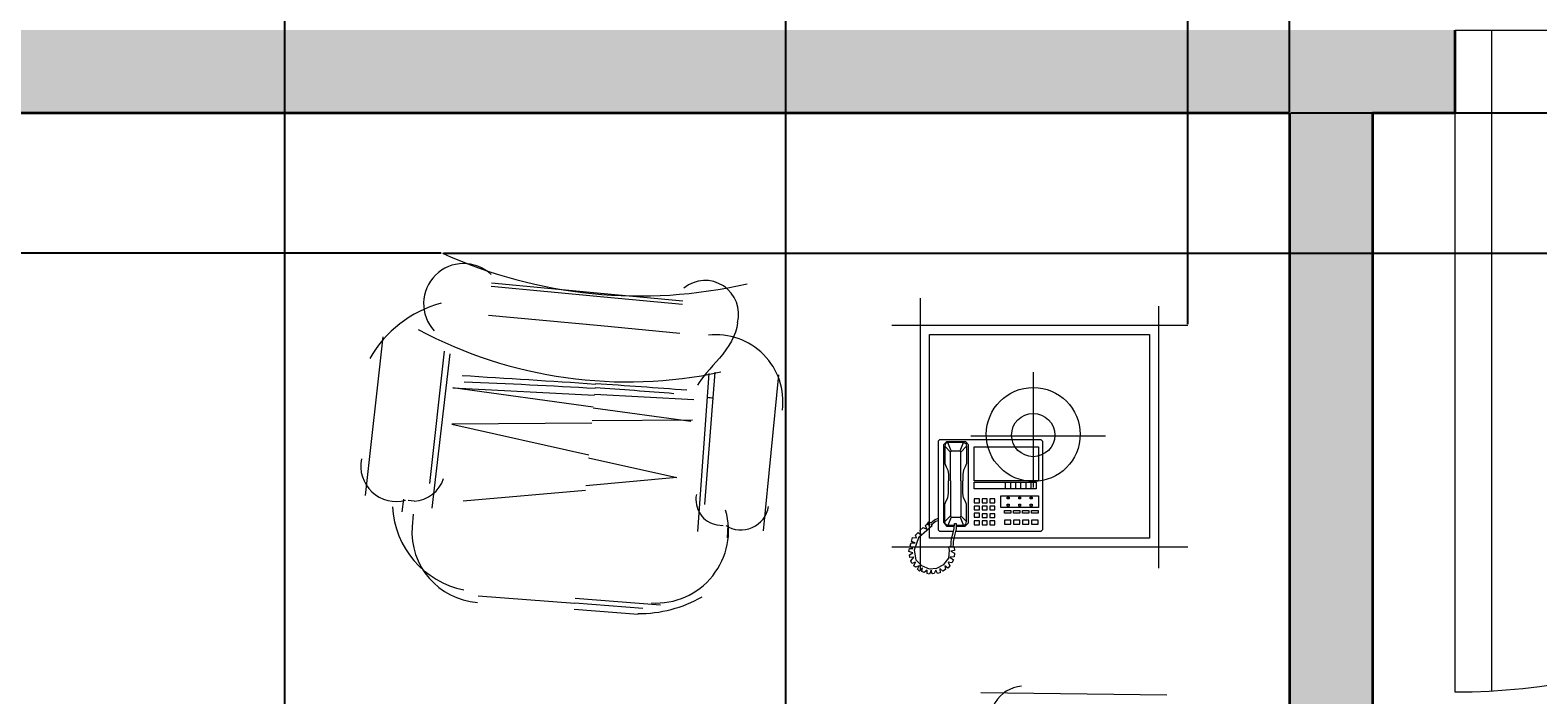
# Model space of a CAD drawing. Units: inches. Extents: x 2807 to 3326, y 2005 to 2580.
# Tile 6 of 12: x 3067 to 3149, y 2243 to 2280. Entities that reach past the tile are written whole.
import ezdxf

# ---------------------------------------------------------------- set-up
doc = ezdxf.new("R2010")
doc.units = ezdxf.units.IN
doc.header["$LTSCALE"] = 0.4
for name, color, linetype, lineweight in [('A-ANNO-DIMS', 2, 'Continuous', 18), ('A-WALL-PATT', 231, 'Continuous', 13), ('DOORS', 144, 'Continuous', 18), ('Furniture', 7, 'Continuous', 15), ('WALL', 233, 'Continuous', 35)]:
    doc.layers.add(name, color=color, linetype=linetype, lineweight=lineweight)
doc.styles.get("Standard").update_dxf_attribs({"font": 'txt', "height": 5})
doc.dimstyles.get("Standard").update_dxf_attribs({"dimtxt": 0.18, "dimasz": 0.18, "dimexe": 0.18, "dimexo": 0.0625, "dimgap": 0.09, "dimtad": 0, "dimtih": 1, "dimtoh": 1, "dimdec": 4, "dimzin": 0, "dimdsep": 46, "dimtxsty": 'Standard', "dimcen": 0.09, "dimadec": 0, "dimazin": 0, "dimtfac": 1, "dimtdec": 4, "dimtofl": 0, "dimtmove": 0, "dimatfit": 3, "dimfxl": 1, "dimtolj": 1, "dimtzin": 0, "dimarcsym": 0})

# ---------------------------------------------------------------- blocks, each defined once
blk = doc.blocks.new('DOOR-36')
for p, q in [((0, 0), (-36, 0)), ((-2, -35.944), (-2, 0)), ((0, -36), (0, 0))]:
    blk.add_line(p, q)
blk.add_arc((0, 0), 36, 180, 270)
blk = doc.blocks.new('*D61')
at = {"layer": 'A-ANNO-DIMS', "color": 0, "lineweight": -2, "ltscale": 0.4, "transparency": 16777216}
for p, q in [((3088.922898, 2267.452063), (2816.937191, 2267.452063)), ((2817.117191, 2267.272063), (2817.117191, 2223.175564)), ((2817.117191, 2173.899065), (2817.117191, 2217.995564)), ((3079.479513, 2173.719065), (2816.937191, 2173.719065))]:
    blk.add_line(p, q, dxfattribs=at)
at = {"layer": 'A-ANNO-DIMS', "color": 0, "ltscale": 0.4, "transparency": 16777216}
for points in [[(2817.087191, 2267.272063), (2817.147191, 2267.272063), (2817.117191, 2267.452063)], [(2817.087191, 2173.899065), (2817.147191, 2173.899065), (2817.117191, 2173.719065)]]:
    blk.add_solid(points, dxfattribs=at)
at = {"layer": 'Defpoints', "color": 0, "ltscale": 0.4, "transparency": 16777216}
for p in [(2817.117191, 2267.452063), (3088.985398, 2267.452063), (3079.542013, 2173.719065)]:
    blk.add_point(p, dxfattribs=at)
at = {"layer": 'A-ANNO-DIMS', "color": 0, "ltscale": 0.4, "transparency": 16777216, "insert": (2817.117191, 2220.585564), "char_height": 5, "attachment_point": 5}
blk.add_mtext('\\A1;93.73', dxfattribs=at)
blk = doc.blocks.new('*D64')
at = {"layer": 'A-ANNO-DIMS', "color": 0, "lineweight": -2, "ltscale": 0.4, "transparency": 16777216}
for p, q in [((3080.426, 2237.614), (3080.426, 2577.206)), ((3080.606, 2577.026), (3081.577, 2577.026)), ((3107.489, 2577.026), (3106.519, 2577.026)), ((3107.669, 2237.614), (3107.669, 2577.206))]:
    blk.add_line(p, q, dxfattribs=at)
at = {"layer": 'A-ANNO-DIMS', "color": 0, "ltscale": 0.4, "transparency": 16777216}
for points in [[(3080.606, 2577.056), (3080.606, 2576.996), (3080.426, 2577.026)], [(3107.489, 2577.056), (3107.489, 2576.996), (3107.669, 2577.026)]]:
    blk.add_solid(points, dxfattribs=at)
at = {"layer": 'Defpoints', "color": 0, "ltscale": 0.4, "transparency": 16777216}
for p in [(3107.669, 2577.026), (3080.426, 2237.552), (3107.669, 2237.552)]:
    blk.add_point(p, dxfattribs=at)
at = {"layer": 'A-ANNO-DIMS', "color": 0, "ltscale": 0.4, "transparency": 16777216, "insert": (3094.048, 2577.026), "char_height": 5, "attachment_point": 5}
blk.add_mtext('\\A1;27.243', dxfattribs=at)
blk = doc.blocks.new('*D66')
at = {"layer": 'A-ANNO-DIMS', "color": 0, "lineweight": -2, "ltscale": 0.4, "transparency": 16777216}
for p, q in [((3129.534988, 2263.581941), (3129.534988, 2577.206496)), ((3129.714988, 2577.026496), (3134.887191, 2577.026496)), ((3135.067191, 2275.138996), (3135.067191, 2577.206496)), ((3135.067191, 2577.026496), (3135.247191, 2577.026496))]:
    blk.add_line(p, q, dxfattribs=at)
at = {"layer": 'A-ANNO-DIMS', "color": 0, "ltscale": 0.4, "transparency": 16777216}
for points in [[(3129.714988, 2577.056496), (3129.714988, 2576.996496), (3129.534988, 2577.026496)], [(3134.887191, 2577.056496), (3134.887191, 2576.996496), (3135.067191, 2577.026496)]]:
    blk.add_solid(points, dxfattribs=at)
at = {"layer": 'Defpoints', "color": 0, "ltscale": 0.4, "transparency": 16777216}
for p in [(3135.067191, 2577.026496), (3135.067191, 2275.076496), (3129.534988, 2263.519441)]:
    blk.add_point(p, dxfattribs=at)
at = {"layer": 'A-ANNO-DIMS', "color": 0, "ltscale": 0.4, "transparency": 16777216, "insert": (3145.337191, 2577.026496), "char_height": 5, "attachment_point": 5}
blk.add_mtext('\\A1;5.532', dxfattribs=at)
blk = doc.blocks.new('*D67')
at = {"layer": 'A-ANNO-DIMS', "color": 0, "lineweight": -2, "ltscale": 0.4, "transparency": 16777216}
for p, q in [((3135.13, 2275.076), (3316.197, 2275.076)), ((3316.017, 2274.896), (3316.017, 2273.854)), ((3316.017, 2267.632), (3316.017, 2268.674)), ((3089.048, 2267.452), (3316.197, 2267.452))]:
    blk.add_line(p, q, dxfattribs=at)
at = {"layer": 'A-ANNO-DIMS', "color": 0, "ltscale": 0.4, "transparency": 16777216}
for points in [[(3315.987, 2274.896), (3316.047, 2274.896), (3316.017, 2275.076)], [(3315.987, 2267.632), (3316.047, 2267.632), (3316.017, 2267.452)]]:
    blk.add_solid(points, dxfattribs=at)
at = {"layer": 'Defpoints', "color": 0, "ltscale": 0.4, "transparency": 16777216}
for p in [(3135.067, 2275.076), (3088.985, 2267.452), (3316.017, 2267.452)]:
    blk.add_point(p, dxfattribs=at)
at = {"layer": 'A-ANNO-DIMS', "color": 0, "ltscale": 0.4, "transparency": 16777216, "insert": (3316.017, 2271.264), "char_height": 5, "attachment_point": 5}
blk.add_mtext('\\A1;7.624', dxfattribs=at)
blk = doc.blocks.new('*D72')
at = {"layer": 'A-ANNO-DIMS', "color": 0, "lineweight": -2, "ltscale": 0.4, "transparency": 16777216}
for p, q in [((2948.067, 2279.639), (2948.067, 2307.206)), ((2948.247, 2307.026), (3060.049, 2307.026)), ((3184.887, 2307.026), (3073.086, 2307.026)), ((3185.067, 2279.639), (3185.067, 2307.206))]:
    blk.add_line(p, q, dxfattribs=at)
at = {"layer": 'A-ANNO-DIMS', "color": 0, "ltscale": 0.4, "transparency": 16777216}
for points in [[(2948.247, 2307.056), (2948.247, 2306.996), (2948.067, 2307.026)], [(3184.887, 2307.056), (3184.887, 2306.996), (3185.067, 2307.026)]]:
    blk.add_solid(points, dxfattribs=at)
at = {"layer": 'Defpoints', "color": 0, "ltscale": 0.4, "transparency": 16777216}
for p in [(3185.067, 2307.026), (2948.067, 2279.576), (3185.067, 2279.576)]:
    blk.add_point(p, dxfattribs=at)
at = {"layer": 'A-ANNO-DIMS', "color": 0, "ltscale": 0.4, "transparency": 16777216, "insert": (3066.567, 2307.026), "char_height": 5, "attachment_point": 5}
blk.add_mtext('\\A1;237', dxfattribs=at)

msp = doc.modelspace()

# ---------------------------------------------------------------- hatches: boundary and pattern name
at = {"layer": 'A-WALL-PATT', "ltscale": 0.4}
h = msp.add_hatch(color=256, dxfattribs=at)
h.dxf.hatch_style = 1
h.paths.add_polyline_path([(3288.5672, 2549.5765), (2941.5672, 2549.5765), (2941.5672, 2540.5765), (2993.5672, 2540.5765), (2993.5672, 2489.5693), (2998.0672, 2489.5693), (2998.0672, 2540.5765), (3135.0672, 2540.5765), (3135.0672, 2479.0765), (3139.5672, 2479.0765), (3139.5672, 2540.5765), (3279.5672, 2540.5765), (3279.5672, 2510.5765), (3288.5672, 2510.5765)])
h.paths.add_polyline_path([(2905.5672, 2549.5765), (2844.5672, 2549.5765), (2844.5672, 2445.94), (2853.5672, 2445.94), (2853.5672, 2540.5765), (2905.5672, 2540.5765)])
h.paths.add_polyline_path([(2853.5672, 2409.94), (2844.5672, 2409.94), (2844.5672, 2371.3497), (2853.5672, 2371.3497), (2853.5672, 2380.0765), (2909.0672, 2380.0765), (2909.0672, 2384.5765), (2853.5672, 2384.5765)])
h.paths.add_polyline_path([(2998.0672, 2389.0765), (2993.5672, 2389.0765), (2993.5672, 2384.5765), (2939.0672, 2384.5765), (2939.0672, 2380.0765), (2943.5672, 2380.0765), (2943.5672, 2314.0765), (2948.0672, 2314.0765), (2948.0672, 2380.0765), (2998.0672, 2380.0765)])
h.paths.add_polyline_path([(2998.0672, 2471.8029), (2993.5672, 2471.8029), (2993.5672, 2425.0765), (2998.0672, 2425.0765)])
h.paths.add_polyline_path([(2953.0672, 2279.5765), (2948.0672, 2279.5765), (2948.0672, 2284.0765), (2943.5672, 2284.0765), (2943.5672, 2279.5765), (2853.5672, 2279.5765), (2853.5672, 2289.0663), (2844.5672, 2289.0663), (2844.5672, 2227.8961), (2853.5672, 2227.8961), (2853.5672, 2275.0765), (2953.0672, 2275.0765)])
h.paths.add_polyline_path([(2943.5672, 2332.0765), (2853.5672, 2332.0765), (2853.5672, 2347.3497), (2844.5672, 2347.3497), (2844.5672, 2313.0663), (2853.5672, 2313.0663), (2853.5672, 2327.5765), (2943.5672, 2327.5765)])
h.paths.add_polyline_path([(3144.0672, 2279.5765), (2993.5672, 2279.5765), (2989.0672, 2279.5765), (2989.0672, 2275.0765), (2993.5672, 2275.0765), (2993.5672, 2144.5765), (2984.5672, 2144.5765), (2984.5672, 2135.5765), (2993.5672, 2135.5765), (2993.5672, 2120.0765), (3036.5672, 2120.0765), (3036.5672, 2129.0765), (2998.0672, 2129.0765), (2998.0672, 2275.0765), (3135.0672, 2275.0765), (3135.0672, 2129.0765), (3096.5672, 2129.0765), (3096.5672, 2120.0765), (3139.5672, 2120.0765), (3139.5672, 2135.5765), (3148.5672, 2135.5765), (3148.5672, 2144.5765), (3139.5672, 2144.5765), (3139.5672, 2275.0765), (3144.0672, 2275.0765)])
h.paths.add_polyline_path([(2984.5672, 2144.5765), (2925.9914, 2144.5765), (2925.9914, 2135.5765), (2984.5672, 2135.5765)])
h.paths.add_polyline_path([(2889.9914, 2144.5765), (2853.5672, 2144.5765), (2853.5672, 2191.8961), (2844.5672, 2191.8961), (2844.5672, 2135.5765), (2889.9914, 2135.5765)])
h.paths.add_polyline_path([(3196.0672, 2144.5765), (3148.5672, 2144.5765), (3148.5672, 2135.5765), (3196.0672, 2135.5765)])
h.paths.add_polyline_path([(3288.5672, 2191.8265), (3279.5672, 2191.8265), (3279.5672, 2144.5765), (3232.0672, 2144.5765), (3232.0672, 2135.5765), (3288.5672, 2135.5765)])
h.paths.add_polyline_path([(3288.5672, 2292.8229), (3279.5672, 2292.8229), (3279.5672, 2291.4371), (3279.5672, 2279.5765), (3189.5672, 2279.5765), (3189.5672, 2293.0765), (3185.0672, 2293.0765), (3185.0672, 2279.5765), (3180.0672, 2279.5765), (3180.0672, 2275.0765), (3279.5672, 2275.0765), (3279.5672, 2227.8265), (3288.5672, 2227.8265)])
h.paths.add_polyline_path([(3288.5672, 2368.0765), (3279.5672, 2368.0765), (3279.5672, 2332.0765), (3174.0672, 2332.0765), (3174.0672, 2327.5765), (3185.0672, 2327.5765), (3189.5672, 2327.5765), (3279.5672, 2327.5765), (3279.5672, 2316.8229), (3288.5672, 2316.8229)])
h.paths.add_polyline_path([(3288.5672, 2474.5765), (3279.5672, 2474.5765), (3279.5672, 2444.5765), (3139.5672, 2444.5765), (3139.5672, 2449.0765), (3135.0672, 2449.0765), (3135.0672, 2327.5765), (3144.0672, 2327.5765), (3144.0672, 2332.0765), (3139.5672, 2332.0765), (3139.5672, 2440.0765), (3279.5672, 2440.0765), (3279.5672, 2404.0765), (3288.5672, 2404.0765)])

# ---------------------------------------------------------------- linework, layer by layer
at = {"layer": 'Furniture'}
for p, q in [((3091.6497, 2265.6621), (3097.7622, 2265.0849)), ((3091.6663, 2265.8372), (3097.7788, 2265.2599)), ((3097.7622, 2265.0849), (3102.0439, 2264.6805)), ((3097.7788, 2265.2599), (3102.0604, 2264.8555)), ((3114.9915, 2250.2169), (3114.9915, 2265.011)), ((3091.5009, 2264.0867), (3097.6134, 2263.5094)), ((3127.942, 2264.5759), (3127.942, 2250.3256)), ((3097.6134, 2263.5094), (3101.8951, 2263.1051)), ((3129.535, 2263.5194), (3113.4239, 2263.5194)), ((3084.8134, 2254.2733), (3085.7585, 2262.9082)), ((3115.4812, 2263.0297), (3127.4523, 2263.0297)), ((3115.4812, 2251.9543), (3115.4812, 2263.0297)), ((3127.4523, 2263.0297), (3127.4523, 2251.9543)), ((3088.3068, 2254.9333), (3089.1099, 2262.121)), ((3088.4292, 2253.5908), (3089.4174, 2261.9813)), ((3102.8876, 2252.3217), (3103.4976, 2260.9089)), ((3103.2691, 2253.7776), (3103.8258, 2260.9885)), ((3107.2595, 2260.8432), (3106.4335, 2252.3569)), ((3121.1232, 2260.9852), (3121.1232, 2254.7047)), ((3097.1952, 2259.0813), (3089.5637, 2260.1318)), ((3089.5637, 2260.1318), (3097.2557, 2259.7216)), ((3097.261, 2259.7772), (3102.6702, 2259.4888)), ((3102.584, 2258.3728), (3097.125, 2258.3374)), ((3102.4914, 2258.2936), (3097.1898, 2259.0233)), ((3097.112, 2258.2001), (3089.4972, 2258.1507)), ((3089.4972, 2258.1507), (3096.9502, 2256.4868)), ((3117.7287, 2257.5259), (3125.0556, 2257.5259)), ((3116.029, 2257.3022), (3115.959, 2257.2323)), ((3115.959, 2257.2323), (3115.959, 2252.4042)), ((3121.5568, 2257.3022), (3116.029, 2257.3022)), ((3116.4138, 2257.1973), (3116.2389, 2257.0223)), ((3116.2389, 2257.0223), (3116.2389, 2252.824)), ((3116.3438, 2257.0923), (3116.3089, 2256.9524)), ((3116.3089, 2256.9524), (3116.6237, 2256.6375)), ((3116.3089, 2256.9524), (3116.3089, 2256.0077)), ((3116.4838, 2257.1623), (3116.3438, 2257.0923)), ((3117.4634, 2257.1973), (3116.4138, 2257.1973)), ((3116.6587, 2256.7075), (3116.4838, 2257.1623)), ((3117.3235, 2257.1623), (3116.4838, 2257.1623)), ((3116.6237, 2256.6375), (3116.6587, 2256.7075)), ((3116.6587, 2256.7075), (3117.1485, 2256.7075)), ((3117.1485, 2256.7075), (3117.3235, 2257.1623)), ((3117.1835, 2256.6375), (3117.1485, 2256.7075)), ((3117.4984, 2256.9524), (3117.1835, 2256.6375)), ((3117.3235, 2257.1623), (3117.4634, 2257.0923)), ((3117.6034, 2257.0223), (3117.4634, 2257.1973)), ((3117.4634, 2257.0923), (3117.4984, 2256.9524)), ((3117.4984, 2256.9524), (3117.4984, 2256.0077)), ((3117.6034, 2252.789), (3117.6034, 2257.0223)), ((3117.9182, 2256.9174), (3121.4169, 2256.9174)), ((3117.9182, 2255.0631), (3117.9182, 2256.9174)), ((3121.4169, 2256.9174), (3121.4169, 2255.0631)), ((3121.5568, 2257.3022), (3121.6268, 2257.2323)), ((3121.6268, 2257.2323), (3121.6268, 2252.4042)), ((3096.934, 2256.3153), (3101.7371, 2255.243)), ((3116.3089, 2256.0077), (3116.3788, 2255.8328)), ((3116.3788, 2255.8328), (3116.4838, 2255.6579)), ((3116.6237, 2255.0631), (3116.6237, 2256.6375)), ((3117.1835, 2255.0631), (3117.1835, 2256.6375)), ((3117.4284, 2255.8328), (3117.3235, 2255.6579)), ((3117.4984, 2256.0077), (3117.4284, 2255.8328)), ((3101.7371, 2255.243), (3096.7911, 2254.8017)), ((3116.4838, 2255.6579), (3116.5188, 2255.413)), ((3116.5188, 2255.413), (3116.5188, 2255.0631)), ((3116.5188, 2254.3984), (3116.5188, 2255.0631)), ((3116.6237, 2255.0631), (3116.6237, 2253.1739)), ((3117.1835, 2255.0631), (3117.1835, 2253.1739)), ((3117.3235, 2255.6579), (3117.2885, 2255.413)), ((3117.2885, 2255.413), (3117.2885, 2255.0631)), ((3117.2885, 2254.3984), (3117.2885, 2255.0631)), ((3121.4169, 2255.0631), (3117.9182, 2255.0631)), ((3096.7673, 2254.5499), (3090.1246, 2253.9572)), ((3116.4838, 2254.1535), (3116.5188, 2254.3984)), ((3117.3235, 2254.1535), (3117.2885, 2254.3984)), ((3117.9182, 2254.9931), (3121.2769, 2254.9931)), ((3117.9182, 2254.6433), (3117.9182, 2254.9931)), ((3121.2769, 2254.6433), (3117.9182, 2254.6433)), ((3119.3527, 2254.2584), (3121.4169, 2254.2584)), ((3119.3527, 2253.6287), (3119.3527, 2254.2584)), ((3119.5976, 2254.9931), (3119.5976, 2254.6433)), ((3119.7025, 2254.0835), (3119.7025, 2254.1885)), ((3119.7025, 2254.1885), (3119.8075, 2254.1885)), ((3119.8075, 2254.1885), (3119.8075, 2254.0835)), ((3119.8775, 2254.9931), (3119.8775, 2254.6433)), ((3120.1573, 2254.9931), (3120.1573, 2254.6433)), ((3120.3323, 2254.0835), (3120.3323, 2254.1885)), ((3120.3323, 2254.1885), (3120.4372, 2254.1885)), ((3120.4372, 2254.9931), (3120.4372, 2254.6433)), ((3120.4372, 2254.1885), (3120.4372, 2254.0835)), ((3120.7171, 2254.9931), (3120.7171, 2254.6433)), ((3120.962, 2254.1885), (3121.067, 2254.1885)), ((3120.962, 2254.0835), (3120.962, 2254.1885)), ((3120.997, 2254.9931), (3120.997, 2254.6433)), ((3121.067, 2254.1885), (3121.067, 2254.0835)), ((3121.2769, 2254.9931), (3121.2769, 2254.6433)), ((3121.4169, 2254.2584), (3121.4169, 2253.6287)), ((3086.8672, 2254.069), (3086.7887, 2253.3893)), ((3087.458, 2253.9711), (3087.1278, 2254.0092)), ((3116.3089, 2253.8036), (3116.3788, 2253.9785)), ((3116.3089, 2252.859), (3116.3089, 2253.8036)), ((3116.3788, 2253.9785), (3116.4838, 2254.1535)), ((3117.4284, 2253.9785), (3117.3235, 2254.1535)), ((3117.4984, 2253.8036), (3117.4284, 2253.9785)), ((3117.4984, 2252.859), (3117.4984, 2253.8036)), ((3118.1981, 2254.0835), (3117.9182, 2254.0835)), ((3117.9182, 2254.0835), (3117.9182, 2253.8736)), ((3117.9182, 2253.8736), (3118.1981, 2253.8736)), ((3117.9182, 2253.6986), (3117.9182, 2253.4887)), ((3118.1981, 2253.6986), (3117.9182, 2253.6986)), ((3117.9182, 2253.4887), (3118.1981, 2253.4887)), ((3118.1981, 2253.8736), (3118.1981, 2254.0835)), ((3118.1981, 2253.4887), (3118.1981, 2253.6986)), ((3118.3381, 2254.0835), (3118.3381, 2253.8736)), ((3118.618, 2254.0835), (3118.3381, 2254.0835)), ((3118.3381, 2253.8736), (3118.618, 2253.8736)), ((3118.3381, 2253.6986), (3118.3381, 2253.4887)), ((3118.618, 2253.6986), (3118.3381, 2253.6986)), ((3118.3381, 2253.4887), (3118.618, 2253.4887)), ((3118.618, 2253.8736), (3118.618, 2254.0835)), ((3118.618, 2253.4887), (3118.618, 2253.6986)), ((3119.0378, 2254.0835), (3118.7579, 2254.0835)), ((3118.7579, 2254.0835), (3118.7579, 2253.8736)), ((3118.7579, 2253.8736), (3119.0378, 2253.8736)), ((3118.7579, 2253.6986), (3118.7579, 2253.4887)), ((3119.0378, 2253.6986), (3118.7579, 2253.6986)), ((3118.7579, 2253.4887), (3119.0378, 2253.4887)), ((3119.0378, 2253.8736), (3119.0378, 2254.0835)), ((3119.0378, 2253.4887), (3119.0378, 2253.6986)), ((3121.4169, 2253.6287), (3119.3527, 2253.6287)), ((3119.5626, 2253.3138), (3119.5626, 2253.4537)), ((3119.5626, 2253.4537), (3119.9124, 2253.4537)), ((3119.8075, 2254.0835), (3119.7025, 2254.0835)), ((3119.7025, 2253.6986), (3119.7025, 2253.8036)), ((3119.7025, 2253.8036), (3119.8075, 2253.8036)), ((3119.8075, 2253.6986), (3119.7025, 2253.6986)), ((3119.8075, 2253.8036), (3119.8075, 2253.6986)), ((3119.9124, 2253.4537), (3119.9124, 2253.3138)), ((3120.0524, 2253.4537), (3120.4023, 2253.4537)), ((3120.0524, 2253.3138), (3120.0524, 2253.4537)), ((3120.4372, 2254.0835), (3120.3323, 2254.0835)), ((3120.3323, 2253.6986), (3120.3323, 2253.8036)), ((3120.3323, 2253.8036), (3120.4372, 2253.8036)), ((3120.4372, 2253.6986), (3120.3323, 2253.6986)), ((3120.4023, 2253.4537), (3120.4023, 2253.3138)), ((3120.4372, 2253.8036), (3120.4372, 2253.6986)), ((3120.5422, 2253.4537), (3120.8921, 2253.4537)), ((3120.5422, 2253.3138), (3120.5422, 2253.4537)), ((3120.8921, 2253.4537), (3120.8921, 2253.3138)), ((3121.067, 2254.0835), (3120.962, 2254.0835)), ((3120.962, 2253.6986), (3120.962, 2253.8036)), ((3120.962, 2253.8036), (3121.067, 2253.8036)), ((3121.067, 2253.6986), (3120.962, 2253.6986)), ((3121.032, 2253.4537), (3121.3819, 2253.4537)), ((3121.032, 2253.3138), (3121.032, 2253.4537)), ((3121.067, 2253.8036), (3121.067, 2253.6986)), ((3121.3819, 2253.4537), (3121.3819, 2253.3138)), ((3087.3925, 2253.2551), (3087.3422, 2252.5728)), ((3087.3925, 2253.2551), (3087.3422, 2252.5728)), ((3103.9227, 2252.6735), (3104.2542, 2252.6491)), ((3104.5214, 2252.6591), (3104.4712, 2251.9768)), ((3115.256, 2252.6413), (3115.3485, 2252.74)), ((3115.33, 2252.4379), (3115.256, 2252.6413)), ((3115.6258, 2252.6228), (3115.3423, 2252.37)), ((3115.3485, 2252.74), (3115.4347, 2252.6722)), ((3115.3854, 2252.777), (3115.4471, 2252.8387)), ((3115.4347, 2252.6722), (3115.3854, 2252.777)), ((3115.4471, 2252.8387), (3115.5765, 2252.7893)), ((3115.5518, 2252.6968), (3115.6258, 2252.6228)), ((3115.6258, 2252.6907), (3115.5518, 2252.6968)), ((3115.5765, 2252.7893), (3115.6504, 2252.8572)), ((3115.6627, 2252.74), (3115.6258, 2252.6907)), ((3115.6504, 2252.8572), (3115.749, 2252.9558)), ((3115.8045, 2252.851), (3115.6627, 2252.74)), ((3115.749, 2252.9558), (3115.959, 2253.0339)), ((3115.959, 2252.894), (3115.8045, 2252.851)), ((3116.2389, 2252.824), (3116.4138, 2252.6141)), ((3116.3089, 2252.859), (3116.6237, 2253.1739)), ((3116.3438, 2252.719), (3116.3089, 2252.859)), ((3116.4838, 2252.6491), (3116.3438, 2252.719)), ((3116.4138, 2252.6141), (3116.8235, 2252.6141)), ((3116.6587, 2253.1039), (3116.4838, 2252.6491)), ((3116.8261, 2252.6491), (3116.4838, 2252.6491)), ((3116.6237, 2253.1739), (3116.6587, 2253.1039)), ((3116.6587, 2253.1039), (3117.1485, 2253.1039)), ((3116.8134, 2252.4736), (3116.8337, 2252.754)), ((3116.8337, 2252.754), (3116.9386, 2252.754)), ((3116.9386, 2252.754), (3116.9337, 2252.4523)), ((3116.9363, 2252.6141), (3117.4284, 2252.6141)), ((3117.3235, 2252.6491), (3116.9369, 2252.6491)), ((3117.1835, 2253.1739), (3117.1485, 2253.1039)), ((3117.1485, 2253.1039), (3117.3235, 2252.6491)), ((3117.4984, 2252.859), (3117.1835, 2253.1739)), ((3117.3235, 2252.6491), (3117.4634, 2252.719)), ((3117.4284, 2252.6141), (3117.6034, 2252.789)), ((3117.4634, 2252.719), (3117.4984, 2252.859)), ((3118.1981, 2253.3138), (3117.9182, 2253.3138)), ((3117.9182, 2253.3138), (3117.9182, 2253.1039)), ((3117.9182, 2253.1039), (3118.1981, 2253.1039)), ((3118.1981, 2252.894), (3117.9182, 2252.894)), ((3117.9182, 2252.894), (3117.9182, 2252.684)), ((3117.9182, 2252.684), (3118.1981, 2252.684)), ((3118.1981, 2253.1039), (3118.1981, 2253.3138)), ((3118.1981, 2252.684), (3118.1981, 2252.894)), ((3118.618, 2253.2788), (3118.3381, 2253.2788)), ((3118.3381, 2253.2788), (3118.3381, 2253.0689)), ((3118.3381, 2253.0689), (3118.618, 2253.0689)), ((3118.618, 2252.894), (3118.3381, 2252.894)), ((3118.3381, 2252.894), (3118.3381, 2252.684)), ((3118.3381, 2252.684), (3118.618, 2252.684)), ((3118.618, 2253.0689), (3118.618, 2253.2788)), ((3118.618, 2252.684), (3118.618, 2252.894)), ((3119.0378, 2253.2788), (3118.7579, 2253.2788)), ((3118.7579, 2253.2788), (3118.7579, 2253.0689)), ((3118.7579, 2253.0689), (3119.0378, 2253.0689)), ((3119.0378, 2252.894), (3118.7579, 2252.894)), ((3118.7579, 2252.894), (3118.7579, 2252.684)), ((3118.7579, 2252.684), (3119.0378, 2252.684)), ((3119.0378, 2253.0689), (3119.0378, 2253.2788)), ((3119.0378, 2252.684), (3119.0378, 2252.894)), ((3119.9124, 2253.3138), (3119.5626, 2253.3138)), ((3119.9124, 2252.929), (3119.5626, 2252.929)), ((3119.5626, 2252.929), (3119.5626, 2252.719)), ((3119.5626, 2252.719), (3119.9124, 2252.719)), ((3119.9124, 2252.719), (3119.9124, 2252.929)), ((3120.4023, 2253.3138), (3120.0524, 2253.3138)), ((3120.0524, 2252.929), (3120.0524, 2252.719)), ((3120.4023, 2252.929), (3120.0524, 2252.929)), ((3120.0524, 2252.719), (3120.4023, 2252.719)), ((3120.4023, 2252.719), (3120.4023, 2252.929)), ((3120.8921, 2253.3138), (3120.5422, 2253.3138)), ((3120.5422, 2252.929), (3120.5422, 2252.719)), ((3120.8921, 2252.929), (3120.5422, 2252.929)), ((3120.5422, 2252.719), (3120.8921, 2252.719)), ((3120.8921, 2252.719), (3120.8921, 2252.929)), ((3121.3819, 2253.3138), (3121.032, 2253.3138)), ((3121.032, 2252.929), (3121.032, 2252.719)), ((3121.3819, 2252.929), (3121.032, 2252.929)), ((3121.032, 2252.719), (3121.3819, 2252.719)), ((3121.3819, 2252.719), (3121.3819, 2252.929)), ((3114.4981, 2251.7722), (3114.5618, 2251.9847)), ((3114.7034, 2251.6942), (3114.4981, 2251.7722)), ((3114.5618, 2251.9847), (3114.7742, 2251.9635)), ((3114.8734, 2251.9635), (3114.6397, 2251.2975)), ((3114.7199, 2252.1172), (3114.8555, 2252.259)), ((3114.7753, 2251.963), (3114.7199, 2252.1172)), ((3114.8555, 2252.259), (3115.0157, 2252.1604)), ((3115.3423, 2252.37), (3114.8801, 2251.9754)), ((3114.9787, 2252.3824), (3115.1389, 2252.5365)), ((3115.0157, 2252.1604), (3114.9787, 2252.3824)), ((3115.1389, 2252.5365), (3115.33, 2252.4379)), ((3127.4523, 2251.9543), (3115.4812, 2251.9543)), ((3115.959, 2252.4042), (3116.029, 2252.3342)), ((3116.029, 2252.3342), (3116.7829, 2252.3342)), ((3116.6576, 2251.7438), (3116.6788, 2251.9139)), ((3116.6647, 2251.5596), (3116.6576, 2251.7438)), ((3116.6788, 2251.9139), (3116.7638, 2252.2469)), ((3116.7638, 2252.2469), (3116.8134, 2252.4736)), ((3116.8488, 2252.0981), (3116.7638, 2251.7651)), ((3116.7638, 2251.7651), (3116.7709, 2251.5809)), ((3116.9337, 2252.4523), (3116.8488, 2252.0981)), ((3116.9054, 2252.3342), (3121.5568, 2252.3342)), ((3121.6268, 2252.4042), (3121.5568, 2252.3342)), ((3129.535, 2251.4646), (3113.4239, 2251.4646)), ((3114.3494, 2251.2196), (3114.3848, 2251.3967)), ((3114.5689, 2251.1558), (3114.3494, 2251.2196)), ((3114.3848, 2251.3967), (3114.576, 2251.3967)), ((3114.3848, 2251.0495), (3114.5689, 2251.1558)), ((3114.4131, 2250.9078), (3114.3848, 2251.0495)), ((3114.6326, 2250.9149), (3114.4131, 2250.9078)), ((3114.4273, 2251.5384), (3114.4769, 2251.7013)), ((3114.576, 2251.3967), (3114.4273, 2251.5384)), ((3114.4627, 2250.7236), (3114.6326, 2250.9149)), ((3114.4769, 2251.7013), (3114.7034, 2251.6942)), ((3114.6397, 2251.2975), (3114.7388, 2250.7661)), ((3116.5301, 2250.8582), (3116.5655, 2251.3046)), ((3116.5372, 2251.4675), (3116.6647, 2251.5596)), ((3116.5655, 2251.3046), (3116.5372, 2251.4675)), ((3116.8204, 2250.9433), (3116.5939, 2250.922)), ((3116.5939, 2250.922), (3116.7921, 2250.7661)), ((3116.8417, 2251.2904), (3116.6363, 2251.255)), ((3116.6363, 2251.255), (3116.8346, 2251.1345)), ((3116.7709, 2251.5809), (3116.7496, 2251.5384)), ((3116.7496, 2251.5384), (3116.8275, 2251.4604)), ((3116.8346, 2251.1345), (3116.8204, 2250.9433)), ((3116.8275, 2251.4604), (3116.8417, 2251.2904)), ((3114.5193, 2250.5819), (3114.4627, 2250.7236)), ((3114.7247, 2250.6457), (3114.5193, 2250.5819)), ((3114.6255, 2250.4544), (3114.7247, 2250.6457)), ((3114.7176, 2250.3694), (3114.6255, 2250.4544)), ((3114.9158, 2250.4544), (3114.7176, 2250.3694)), ((3114.7388, 2250.7661), (3115.0504, 2250.4615)), ((3114.8309, 2250.2631), (3114.9158, 2250.4544)), ((3114.9442, 2250.1639), (3114.8309, 2250.2631)), ((3115.0928, 2250.3481), (3114.9442, 2250.1639)), ((3115.0504, 2250.4615), (3115.461, 2250.2844)), ((3115.0716, 2250.1356), (3115.0928, 2250.3481)), ((3115.1849, 2250.0789), (3115.0716, 2250.1356)), ((3115.3477, 2250.2206), (3115.1849, 2250.0789)), ((3115.3548, 2250.0293), (3115.3477, 2250.2206)), ((3115.461, 2250.2844), (3115.8858, 2250.3198)), ((3115.5672, 2250.2206), (3115.4893, 2249.9939)), ((3115.6168, 2250.0152), (3115.5672, 2250.2206)), ((3115.8221, 2250.2206), (3115.7372, 2250.0293)), ((3115.9142, 2250.0293), (3115.8221, 2250.2206)), ((3115.8858, 2250.3198), (3116.2611, 2250.5182)), ((3116.0416, 2250.3056), (3116.0628, 2250.0718)), ((3116.2115, 2250.1639), (3116.0416, 2250.3056)), ((3116.3461, 2250.249), (3116.2115, 2250.1639)), ((3116.2611, 2250.5182), (3116.5301, 2250.8582)), ((3116.3177, 2250.4402), (3116.3461, 2250.249)), ((3116.4806, 2250.3198), (3116.3177, 2250.4402)), ((3116.5868, 2250.4473), (3116.4806, 2250.3198)), ((3116.4877, 2250.6457), (3116.5868, 2250.4473)), ((3116.7001, 2250.6032), (3116.4877, 2250.6457)), ((3116.7921, 2250.7661), (3116.7001, 2250.6032)), ((3115.4893, 2249.9939), (3115.3548, 2250.0293)), ((3115.7372, 2250.0293), (3115.6168, 2250.0152)), ((3116.0628, 2250.0718), (3115.9142, 2250.0293)), ((3096.1859, 2248.3942), (3090.9369, 2248.7995)), ((3100.8565, 2248.3162), (3096.2124, 2248.6747)), ((3099.6439, 2247.8101), (3096.1561, 2248.0784)), ((3099.8912, 2248.1316), (3096.1881, 2248.4175)), ((3118.269, 2243.56), (3128.3948, 2243.4339))]:
    msp.add_line(p, q, dxfattribs=at)
for centre, radius in [((3121.1232, 2257.593), 2.5525), ((3121.1232, 2257.5595), 1.1755)]:
    msp.add_circle(centre, radius, dxfattribs=at)
for centre, radius, start, end in [((3099.7264, 2291.0591), 25.9357, 245.534854, 283.001205), ((3090.1398, 2264.7096), 2.1745, 46.591864, 222.74892), ((3103.2764, 2264.1449), 1.82, 344.590834, 129.179615), ((3090.5689, 2258.5753), 6.3658, 105.055783, 150.338961), ((3099.0594, 2284.646), 24.1942, 241.939753, 282.111286), ((3103.8859, 2259.3848), 3.6236, 352.651511, 96.805054), ((3032.7009, 1306.6529), 955.851, 86.1241132, 86.5591928), ((3079.3031, 1967.4569), 293.179, 86.482641, 87.874142), ((3077.9433, 1967.5853), 293.179, 85.374917, 86.215594), ((3031.3411, 1306.7814), 955.851, 85.7441098, 86.0422152), ((3062.261, 1969.3238), 293.179, 81.871375, 81.933336), ((3086.4641, 2255.8684), 1.9154, 168.010079, 285.815494), ((3087.3613, 2255.7449), 1.7765, 273.119298, 342.107634), ((3104.1758, 2254.0523), 1.4018, 169.02937, 259.596142), ((3091.1262, 2253.8917), 4.8525, 182.698589, 258.541474), ((3100.607, 2252.3669), 3.9444, 266.424998, 16.294311), ((3105.2212, 2253.9183), 1.5224, 237.195546, 350.985493), ((3091.1706, 2252.291), 3.8387, 175.790439, 265.790439), ((3099.6464, 2254.8611), 7.013, 269.801493, 299.573326), ((3120.6643, 2242.0094), 1.9033, 95.650869, 200.597543)]:
    msp.add_arc(centre, radius, start, end, dxfattribs=at)
msp.add_open_spline([(3105.031, 2263.6613), (3104.9233, 2262.2658), (3103.2735, 2261.0884), (3102.866, 2260.267)], degree=3, dxfattribs=at)
at = {"layer": 'WALL'}
for p, q in [((3144.0672, 2275.0765), (3144.0672, 2279.5765)), ((2998.0672, 2275.0765), (3135.0672, 2275.0765)), ((3135.0672, 2275.0765), (3135.0672, 2129.0765)), ((3139.5672, 2275.0765), (3139.5672, 2144.5765)), ((3139.5672, 2275.0765), (3144.0672, 2275.0765))]:
    msp.add_line(p, q, dxfattribs=at)

# ---------------------------------------------------------------- block references
at = {"layer": 'DOORS', "extrusion": (0, 0, -1), "zscale": -1}
msp.add_blockref('DOOR-36', (-3144.0672, 2279.5765), dxfattribs=at)

# ---------------------------------------------------------------- dimensions: what is measured, and where the dimension line sits
at = {"layer": 'A-ANNO-DIMS', "ltscale": 0.4}
for base, p1, p2, picture, middle in [((3107.6694, 2577.0265), (3080.4262, 2237.5518), (3107.6694, 2237.5518), '*D64', (3094.0478, 2577.0265)), ((3135.0672, 2577.0265), (3129.535, 2263.5194), (3135.0672, 2275.0765), '*D66', (3145.3372, 2577.0265))]:
    dim = msp.add_linear_dim(base=base, p1=p1, p2=p2, dimstyle='Standard', override={"dimdec": 3, "dimlfac": 1, "dimrnd": 0, "dimzin": 0, "dimdsep": 46, "dimlunit": 2}, dxfattribs=at)
    dim.commit()
    dim.dimension.update_dxf_attribs({"geometry": picture, "text_midpoint": middle})
for base, p1, p2, angle, override, picture, middle in [((3185.0672, 2307.0265), (2948.0672, 2279.5765), (3185.0672, 2279.5765), 0, {"dimdec": 0, "dimlfac": 1, "dimrnd": 0, "dimzin": 0, "dimdsep": 46, "dimlunit": 2}, '*D72', (3066.5672, 2307.0265)), ((3316.0172, 2267.4521), (3135.0672, 2275.0765), (3088.9854, 2267.4521), 90, {"dimdec": 3, "dimlfac": 1, "dimrnd": 0, "dimzin": 0, "dimdsep": 46, "dimlunit": 2}, '*D67', (3316.0172, 2271.2643)), ((2817.1172, 2267.4521), (3079.542, 2173.7191), (3088.9854, 2267.4521), 90, {"dimdec": 2, "dimlfac": 1, "dimrnd": 0, "dimzin": 0, "dimdsep": 46, "dimlunit": 2}, '*D61', (2817.1172, 2220.5856))]:
    dim = msp.add_linear_dim(base=base, p1=p1, p2=p2, angle=angle, dimstyle='Standard', override=override, dxfattribs=at)
    dim.commit()
    dim.dimension.update_dxf_attribs({"geometry": picture, "text_midpoint": middle})

doc.saveas('drawing.dxf')
